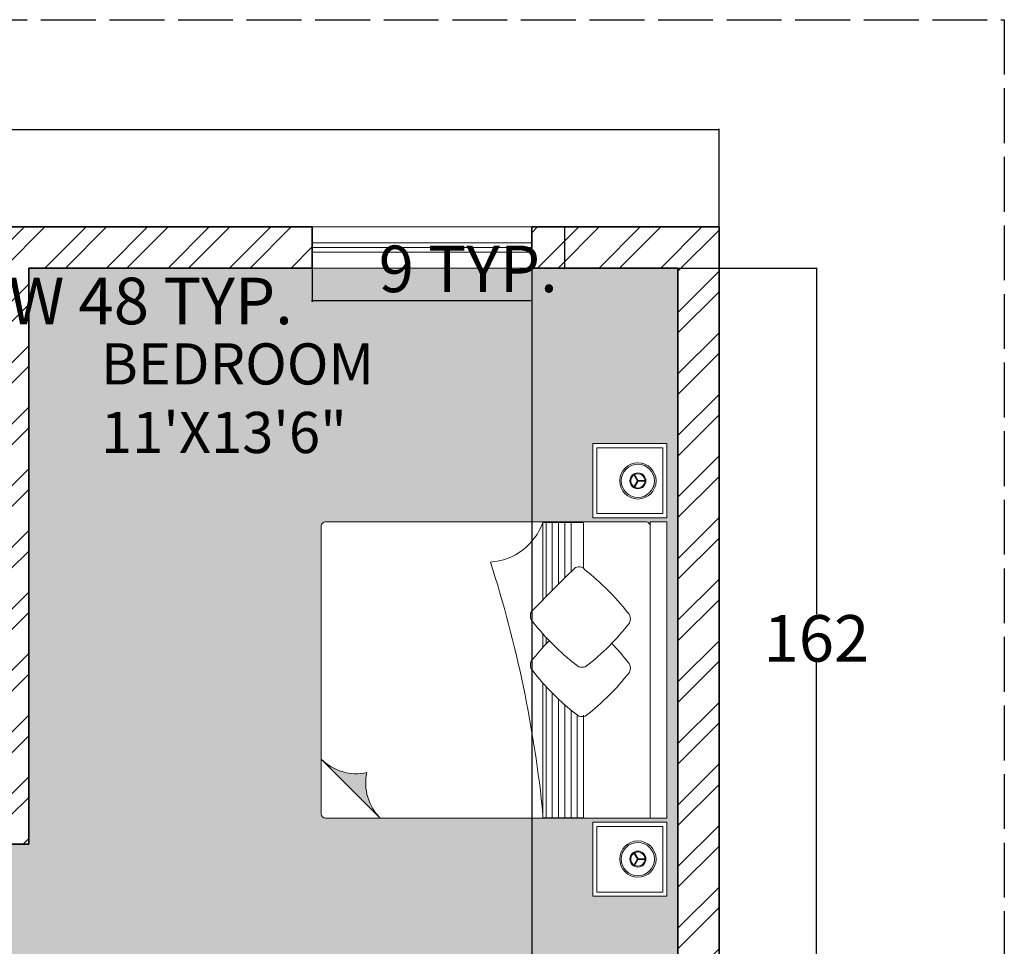
# Model space of a CAD drawing. Units: inches. Extents: x 1410 to 1959, y 5441 to 5968.
# Tile 5 of 5: x 1705 to 1920, y 5765 to 5968. Entities that reach past the tile are written whole.
import ezdxf

# ---------------------------------------------------------------- set-up
doc = ezdxf.new("R2010")
doc.units = ezdxf.units.IN
doc.linetypes.add('ACAD_ISO02W100', pattern=[15, 12, -3])
doc.layers.get('Defpoints').update_dxf_attribs({"linetype": 'ACAD_ISO02W100'})
for name, color, linetype, lineweight in [('00 FURNITURE', 15, 'Continuous', 15), ('A-ANNO-DIMS', 2, 'Continuous', 18), ('A-AREA-IDEN', 7, 'Continuous', 18), ('A-WALL', 7, 'Continuous', 35), ('A-WALL-PATT', 8, 'Continuous', 13), ('WINDOW', 160, 'Continuous', 13)]:
    doc.layers.add(name, color=color, linetype=linetype, lineweight=lineweight)
doc.layers.add('A-FLOR-PATT', color=9, linetype='Continuous', lineweight=9, true_color=0xafd9aa)
doc.styles.get("Standard").update_dxf_attribs({"font": 'arial.ttf'})
doc.dimstyles.get("Standard").update_dxf_attribs({"dimtxt": 10.18, "dimasz": 0.18, "dimexe": 0.18, "dimexo": 0.0625, "dimgap": 0.09, "dimtad": 0, "dimtih": 1, "dimtoh": 1, "dimdec": 0, "dimzin": 0, "dimdsep": 46, "dimlunit": 3, "dimtxsty": 'Standard', "dimcen": 0.09, "dimadec": 0, "dimazin": 0, "dimtfac": 1, "dimtdec": 0, "dimtofl": 0, "dimtmove": 0, "dimatfit": 3, "dimfxl": 1, "dimtolj": 1, "dimtzin": 0, "dimarcsym": 0})

# ---------------------------------------------------------------- blocks, each defined once
blk = doc.blocks.new('RGWTG')
at = {"layer": '00 FURNITURE'}
for p, q in [((578.23, 3473.51), (577.36, 3475.01)), ((578.36, 3473.58), (577.49, 3475.09)), ((578.23, 3473.58), (577.36, 3472.08)), ((578.36, 3473.51), (577.49, 3472)), ((578.29, 3473.62), (580.03, 3473.62)), ((578.29, 3473.47), (580.03, 3473.47)), ((521.93, 3464.58), (509.03, 3451.68)), ((509.03, 3422.63), (509.03, 3463.68)), ((509.93, 3464.58), (566.4, 3464.58)), ((557.53, 3463.84), (557.53, 3464.49)), ((557.53, 3464.49), (566.4, 3464.49)), ((558.2, 3464.49), (558.2, 3435.82)), ((559.57, 3464.49), (559.57, 3437.25)), ((560.94, 3464.49), (560.94, 3438.58)), ((562.3, 3464.49), (562.3, 3439.83)), ((563.67, 3464.49), (563.67, 3440.99)), ((565.04, 3464.49), (565.04, 3442.08)), ((566.4, 3464.58), (580.98, 3464.58)), ((566.4, 3464.49), (566.4, 3442.08)), ((566.4, 3464.49), (566.4, 3463.84)), ((580.98, 3464.58), (580.98, 3416.72)), ((558.2, 3426.48), (558.2, 3425.04)), ((509.03, 3400.68), (509.03, 3422.63)), ((558.2, 3416.13), (558.2, 3399.95)), ((580.98, 3416.72), (580.98, 3400.68)), ((559.57, 3414.75), (559.57, 3399.95)), ((560.94, 3413.39), (560.94, 3399.95)), ((562.3, 3412.04), (562.3, 3399.95)), ((563.67, 3410.72), (563.67, 3399.95)), ((580.08, 3399.78), (509.93, 3399.78)), ((557.53, 3399.95), (557.53, 3400.6)), ((566.4, 3399.95), (557.53, 3399.95)), ((566.4, 3400.6), (566.4, 3399.95)), ((578.23, 3390.78), (577.36, 3392.29)), ((578.36, 3390.86), (577.49, 3392.36)), ((578.23, 3390.86), (577.36, 3389.36)), ((578.36, 3390.78), (577.49, 3389.28)), ((578.29, 3390.9), (580.03, 3390.9)), ((578.29, 3390.74), (580.03, 3390.74))]:
    blk.add_line(p, q, dxfattribs=at)
for points in [[(568.43, 3465.48), (584.63, 3465.48), (584.63, 3481.68), (568.43, 3481.68)], [(569.33, 3466.38), (583.73, 3466.38), (583.73, 3480.78), (569.33, 3480.78)], [(580.98, 3399.78), (584.63, 3399.78), (584.63, 3464.58), (580.98, 3464.58)], [(568.43, 3398.88), (584.63, 3398.88), (584.63, 3382.68), (568.43, 3382.68)], [(569.33, 3397.98), (583.73, 3397.98), (583.73, 3383.58), (569.33, 3383.58)]]:
    blk.add_lwpolyline(points, close=True, dxfattribs=at)
for points in [[(566.52, 3464.49), (557.53, 3464.49), (557.53, 3435.08)], [(557.53, 3427.21), (557.53, 3424.3)], [(557.53, 3416.82), (557.53, 3399.95), (566.4, 3399.95), (566.4, 3409.94)]]:
    blk.add_lwpolyline(points, dxfattribs=at)
for centre, radius in [((578.29, 3473.54), 3.97), ((578.29, 3473.54), 3.63), ((578.29, 3473.54), 1.74), ((578.29, 3473.54), 1.56), ((578.29, 3390.82), 3.97), ((578.29, 3390.82), 3.63), ((578.29, 3390.82), 1.74), ((578.29, 3390.82), 1.56)]:
    blk.add_circle(centre, radius, dxfattribs=at)
for centre, radius, start, end in [((509.93, 3463.68), 0.9, 90, 180), ((529.65, 3456.88), 10.9, 135.0361, 191.9278), ((290.56, 3490.52), 268.3, 342.2214, 354.2925), ((516.73, 3443.97), 10.9, 78.0722, 134.9639), ((598.15, 3399.01), 54.32, 127.931, 142.069), ((566.05, 3440.57), 1.82, 45, 135), ((533.58, 3399.31), 54.32, 37.931, 52.069), ((556.59, 3431.11), 1.82, 135, 225), ((598.15, 3388.23), 54.32, 127.931, 142.069), ((566.05, 3429.78), 1.82, 45, 135), ((533.58, 3388.53), 54.32, 37.931, 52.069), ((574.84, 3431.77), 1.82, 315, 45), ((597.87, 3463.6), 54.32, 217.931, 224.141), ((533.28, 3463.88), 54.32, 316.32, 322.069), ((556.59, 3420.33), 1.82, 135, 225), ((574.84, 3420.99), 1.82, 315, 45), ((765.33, 3619.75), 290.45, 223.6069, 226.2326), ((533.28, 3453.1), 54.32, 307.931, 322.069), ((565.44, 3411.05), 1.47, 225.9674, 326.8337), ((545.02, 3395.29), 13.35, 20.4224, 85.5825), ((509.93, 3400.68), 0.9, 180, 270), ((580.08, 3400.68), 0.9, 270, 0)]:
    blk.add_arc(centre, radius, start, end, dxfattribs=at)
blk = doc.blocks.new('WIN-48IN')
for p, q in [((48, 9), (0, 9)), ((0, 5.5), (48, 5.5)), ((0, 4.5), (48, 4.5)), ((0, 3.5), (48, 3.5)), ((0, 0), (48, 0))]:
    blk.add_line(p, q)
blk = doc.blocks.new('*D10')
at = {"layer": 'A-ANNO-DIMS', "color": 0, "lineweight": -2, "transparency": 16777216}
for p, q in [((1769.1, 5913.3), (1769.1, 5905.99)), ((1817.1, 5913.3), (1817.1, 5905.99)), ((1769.1, 5906.17), (1768.92, 5906.17)), ((1816.92, 5906.17), (1769.28, 5906.17))]:
    blk.add_line(p, q, dxfattribs=at)
at = {"layer": 'A-ANNO-DIMS', "color": 0, "transparency": 16777216}
for points in [[(1769.28, 5906.2), (1769.28, 5906.14), (1769.1, 5906.17)], [(1816.92, 5906.2), (1816.92, 5906.14), (1817.1, 5906.17)]]:
    blk.add_solid(points, dxfattribs=at)
at = {"layer": 'Defpoints', "color": 0, "transparency": 16777216}
for p in [(1769.1, 5913.37), (1817.1, 5913.37), (1769.1, 5906.17)]:
    blk.add_point(p, dxfattribs=at)
at = {"layer": 'A-ANNO-DIMS', "color": 0, "transparency": 16777216, "insert": (1710.67, 5906.17), "char_height": 10.18, "attachment_point": 5}
blk.add_mtext('\\A1;WINDOW 48 TYP.', dxfattribs=at)
blk = doc.blocks.new('*D11')
at = {"layer": 'A-ANNO-DIMS', "color": 0, "lineweight": -2, "transparency": 16777216}
for p, q in [((1817.17, 5922.37), (1824.48, 5922.37)), ((1824.3, 5922.19), (1824.3, 5913.55)), ((1817.17, 5913.37), (1824.48, 5913.37)), ((1824.3, 5913.19), (1824.12, 5913.19)), ((1824.3, 5913.37), (1824.3, 5913.19))]:
    blk.add_line(p, q, dxfattribs=at)
at = {"layer": 'A-ANNO-DIMS', "color": 0, "transparency": 16777216}
for points in [[(1824.27, 5922.19), (1824.33, 5922.19), (1824.3, 5922.37)], [(1824.27, 5913.55), (1824.33, 5913.55), (1824.3, 5913.37)]]:
    blk.add_solid(points, dxfattribs=at)
at = {"layer": 'Defpoints', "color": 0, "transparency": 16777216}
for p in [(1817.1, 5922.37), (1817.1, 5913.37), (1824.3, 5913.37)]:
    blk.add_point(p, dxfattribs=at)
at = {"layer": 'A-ANNO-DIMS', "color": 0, "transparency": 16777216, "insert": (1803.21, 5913.19), "char_height": 10.18, "attachment_point": 5}
blk.add_mtext('\\A1;9 TYP.', dxfattribs=at)
blk = doc.blocks.new('*D24')
at = {"layer": 'A-ANNO-DIMS', "color": 0, "lineweight": -2, "transparency": 16777216}
for p, q in [((1486.09, 5922.43), (1486.09, 5943.8)), ((1486.27, 5943.62), (1660.81, 5943.62)), ((1857.91, 5943.62), (1683.37, 5943.62)), ((1858.09, 5922.43), (1858.09, 5943.8))]:
    blk.add_line(p, q, dxfattribs=at)
at = {"layer": 'A-ANNO-DIMS', "color": 0, "transparency": 16777216}
for points in [[(1486.27, 5943.65), (1486.27, 5943.59), (1486.09, 5943.62)], [(1857.91, 5943.65), (1857.91, 5943.59), (1858.09, 5943.62)]]:
    blk.add_solid(points, dxfattribs=at)
at = {"layer": 'Defpoints', "color": 0, "transparency": 16777216}
for p in [(1858.09, 5943.62), (1486.09, 5922.37), (1858.09, 5922.37)]:
    blk.add_point(p, dxfattribs=at)
at = {"layer": 'A-ANNO-DIMS', "color": 0, "transparency": 16777216, "insert": (1672.09, 5943.62), "char_height": 10.18, "attachment_point": 5}
blk.add_mtext('\\A1;372', dxfattribs=at)
blk = doc.blocks.new('*D28')
at = {"layer": 'A-ANNO-DIMS', "color": 0, "lineweight": -2, "transparency": 16777216}
for p, q in [((1817.1, 5913.3), (1817.1, 5478.87)), ((1849.09, 5913.3), (1849.09, 5478.87)), ((1817.28, 5479.05), (1848.91, 5479.05)), ((1849.09, 5479.05), (1849.27, 5479.05))]:
    blk.add_line(p, q, dxfattribs=at)
at = {"layer": 'A-ANNO-DIMS', "color": 0, "transparency": 16777216}
for points in [[(1817.28, 5479.08), (1817.28, 5479.02), (1817.1, 5479.05)], [(1848.91, 5479.08), (1848.91, 5479.02), (1849.09, 5479.05)]]:
    blk.add_solid(points, dxfattribs=at)
at = {"layer": 'Defpoints', "color": 0, "transparency": 16777216}
for p in [(1817.1, 5913.37), (1849.09, 5913.37), (1849.09, 5479.05)]:
    blk.add_point(p, dxfattribs=at)
at = {"layer": 'A-ANNO-DIMS', "color": 0, "transparency": 16777216, "insert": (1866.55, 5479.05), "char_height": 10.18, "attachment_point": 5}
blk.add_mtext('\\A1;31.99', dxfattribs=at)
blk = doc.blocks.new('*D43')
at = {"layer": 'A-ANNO-DIMS', "color": 0, "lineweight": -2, "transparency": 16777216}
for p, q in [((1849.16, 5913.37), (1879.55, 5913.37)), ((1879.37, 5913.19), (1879.37, 5837.65)), ((1879.37, 5751.55), (1879.37, 5827.08)), ((1849.16, 5751.37), (1879.55, 5751.37))]:
    blk.add_line(p, q, dxfattribs=at)
at = {"layer": 'A-ANNO-DIMS', "color": 0, "transparency": 16777216}
for points in [[(1879.34, 5913.19), (1879.4, 5913.19), (1879.37, 5913.37)], [(1879.34, 5751.55), (1879.4, 5751.55), (1879.37, 5751.37)]]:
    blk.add_solid(points, dxfattribs=at)
at = {"layer": 'Defpoints', "color": 0, "transparency": 16777216}
for p in [(1849.09, 5913.37), (1879.37, 5913.37), (1849.09, 5751.37)]:
    blk.add_point(p, dxfattribs=at)
at = {"layer": 'A-ANNO-DIMS', "color": 0, "transparency": 16777216, "insert": (1879.37, 5832.37), "char_height": 10.18, "attachment_point": 5}
blk.add_mtext('\\A1;162', dxfattribs=at)

msp = doc.modelspace()

# ---------------------------------------------------------------- hatches: boundary and pattern name
at = {"layer": 'A-FLOR-PATT', "transparency": 33554534}
h = msp.add_hatch(color=256, dxfattribs=at)
h.dxf.hatch_style = 1
h.paths.add_polyline_path([(1849.0942, 5913.3659), (1817.1029, 5913.3659), (1769.1029, 5913.3659), (1769.1029, 5913.3659), (1707.0942, 5913.3659), (1707.0942, 5787.3659), (1703.0942, 5787.3659), (1703.0942, 5799.3659), (1631.0942, 5799.3659), (1631.0942, 5787.3659), (1627.0942, 5787.3659), (1627.0942, 5889.3659), (1519.0989, 5889.3659), (1519.0989, 5816.4745), (1495.0981, 5816.4745), (1495.0981, 5809.856), (1495.0942, 5751.3659), (1631.0942, 5751.3659), (1631.0942, 5747.3659), (1495.0942, 5747.3659), (1495.0942, 5702.5811), (1495.0984, 5654.5768), (1495.0942, 5603.3659), (1667.0942, 5603.3659), (1667.0942, 5594.3659), (1650.778, 5594.3659), (1650.778, 5558.3659), (1703.0942, 5558.3659), (1703.0942, 5594.3659), (1703.0942, 5711.3659), (1707.0942, 5711.3659), (1707.0942, 5535.3659), (1754.5413, 5535.3659), (1802.541, 5535.3658), (1802.5413, 5535.3658), (1802.5413, 5535.3659), (1849.0942, 5535.3659), (1849.0942, 5651.3659), (1743.0942, 5651.3659), (1743.0942, 5655.3659), (1849.0942, 5655.3659), (1849.0942, 5665.4579), (1849.0942, 5689.4579), (1849.0942, 5699.3659), (1801.0942, 5699.3659), (1801.0942, 5685.3659), (1797.0942, 5685.3659), (1797.0942, 5699.3659), (1783.0942, 5699.3659), (1783.0942, 5703.3659), (1849.0942, 5703.3659), (1849.0942, 5716.9764), (1849.123, 5716.9764), (1849.123, 5740.9654), (1849.0942, 5740.9654), (1849.0942, 5747.3659), (1753.0942, 5747.3659), (1753.0942, 5699.3659), (1749.0942, 5699.3659), (1749.0942, 5747.3659), (1707.0942, 5747.3659), (1691.0942, 5747.3659), (1691.0942, 5751.3659), (1707.0942, 5751.3659), (1849.0942, 5751.3659)])
h.paths.add_polyline_path([(1533.4842, 5711.1518), (1533.4842, 5637.9201), (1534.7464, 5637.9201), (1534.7464, 5640.1099, -0.41421356), (1536.9363, 5642.2998), (1558.8347, 5642.2998, -0.41421356), (1561.0246, 5640.1099), (1561.0246, 5637.9201), (1563.2144, 5637.9201, -0.41421356), (1565.4042, 5635.7302), (1565.4042, 5609.4519, -0.41421356), (1563.2144, 5607.2621), (1532.5566, 5607.2621, -0.41421356), (1530.3668, 5609.4519), (1530.3668, 5635.4862), (1529.1045, 5635.4862), (1529.1045, 5633.2964, -0.41421356), (1526.9147, 5631.1065), (1500.6363, 5631.1065, -0.41421356), (1498.4465, 5633.2964), (1498.4465, 5715.5315, -0.41421356), (1500.6363, 5717.7213), (1526.9147, 5717.7213, -0.41421356), (1529.1045, 5715.5315), (1529.1045, 5713.3417), (1531.2944, 5713.3417, -0.41421356)], flags=16)
h.paths.add_polyline_path([(1771.0631, 5793.9619), (1771.0631, 5835.0118), (1771.0631, 5856.9619, -0.41421356), (1771.9631, 5857.8619), (1842.1181, 5857.8619, -0.41421356), (1843.0181, 5856.9619), (1843.0181, 5857.8619), (1846.6631, 5857.8619), (1846.6631, 5793.0619), (1843.0181, 5793.0619), (1828.4381, 5793.0619), (1771.9631, 5793.0619, -0.41421356)], flags=16)
h.paths.add_polyline_path([(1771.0631, 5805.9671, 0.25346465), (1781.0166, 5803.0153, 0.25379956), (1783.9781, 5793.0522)], flags=16)
h.paths.add_polyline_path([(1746.3058, 5612.0795), (1768.2559, 5612.0795), (1809.3058, 5612.0795, -0.41421356), (1810.2058, 5611.1795), (1810.2058, 5554.7045), (1810.2058, 5540.1245), (1810.2058, 5536.4795), (1745.4058, 5536.4795), (1745.4058, 5540.1245), (1746.3058, 5540.1245, -0.41421356), (1745.4058, 5541.0245), (1745.4058, 5611.1795, -0.41421356)], flags=16)
h.paths.add_polyline_path([(1819.5646, 5793.1537), (1819.5646, 5793.8054, 0.05271893), (1808.0815, 5849.0458, 0.29223153), (1819.5646, 5857.6981), (1828.4381, 5857.6981), (1828.4381, 5857.0464), (1828.4381, 5847.601, -0.06332793), (1838.1593, 5837.9401, -0.38046479), (1838.3062, 5835.5217, -0.02593615), (1834.5989, 5831.2824, -0.02509022), (1838.1593, 5827.1584, -0.38046478), (1838.3062, 5824.74, -0.05941785), (1829.2061, 5815.646, -0.11763956), (1828.4381, 5815.2914), (1828.4381, 5793.1537)], flags=0)
h.paths.add_polyline_path([(1819.5646, 5793.1537), (1819.5646, 5822.5662, -0.01603557), (1817.3363, 5825.2436, -0.4295765), (1817.4052, 5827.8865, -0.01537126), (1819.5646, 5830.4335), (1819.5646, 5833.3479, -0.01603557), (1817.3363, 5836.0254, -0.48413611), (1817.6682, 5838.8652, 0.00079305), (1817.0318, 5838.199, 0.26524804), (1817.0526, 5836.3926, 0.02736634), (1820.9176, 5831.8795, 0.02734261), (1817.0221, 5827.3996, 0.26229506), (1817.0526, 5825.6108, 0.06555279), (1827.0712, 5815.5721), (1827.0712, 5793.1537)], flags=0)
h.paths.add_polyline_path([(1830.4631, 5775.9619), (1830.4631, 5792.1619), (1846.6631, 5792.1619), (1846.6631, 5775.9619)], flags=16)
h.paths.add_polyline_path([(1831.3631, 5776.8619), (1831.3631, 5791.2619), (1845.7631, 5791.2619), (1845.7631, 5776.8619)], flags=0)
h.paths.add_polyline_path([(1836.6983, 5784.1006, -1), (1843.9547, 5784.1006, -1)], flags=0)
h.paths.add_polyline_path([(1819.2615, 5682.5311, -0.25820517), (1830.2865, 5687.0962, -0.1716359), (1835.799, 5683.9093), (1838.1615, 5683.9093), (1838.1615, 5688.0436, -0.41421356), (1839.1458, 5689.028), (1845.4458, 5689.028, -0.41421356), (1846.4302, 5688.0436), (1846.4302, 5671.8999, -0.41421356), (1845.4458, 5670.9155), (1839.1458, 5670.9155, -0.41421356), (1838.1615, 5671.8999), (1838.1615, 5676.0343), (1835.799, 5676.0343, -0.1716359), (1830.2865, 5672.8474, -0.25820517), (1819.2615, 5677.4124)], flags=16)
h.paths.add_polyline_path([(1820.8043, 5682.5681, -0.21038447), (1830.2865, 5685.5212, -0.1716359), (1835.799, 5682.3343), (1835.799, 5677.6093, -0.1716359), (1830.2865, 5674.4224, -0.21038447), (1820.8043, 5677.3755)], flags=0)
h.paths.add_polyline_path([(1842.0614, 5784.0231), (1841.8811, 5784.0231, -0.54460611), (1839.6163, 5782.7155), (1839.5262, 5782.5594, 0.54796211)], flags=0)
h.paths.add_polyline_path([(1840.3713, 5784.1781), (1840.3265, 5784.2556), (1840.2818, 5784.1781)], flags=0)
h.paths.add_polyline_path([(1830.4631, 5858.7619), (1830.4631, 5874.9619), (1846.6631, 5874.9619), (1846.6631, 5858.7619)], flags=16)
h.paths.add_polyline_path([(1831.3631, 5859.6619), (1831.3631, 5874.0619), (1845.7631, 5874.0619), (1845.7631, 5859.6619)], flags=0)
h.paths.add_polyline_path([(1755.6206, 5556.6903, -0.00089292), (1756.3396, 5557.4382), (1745.5695, 5557.4382), (1745.5695, 5554.7045), (1746.2212, 5554.7045), (1755.5673, 5554.7045, -0.38881883)], flags=0)
h.paths.add_polyline_path([(1810.114, 5563.578), (1810.114, 5554.7045), (1809.4622, 5554.7045), (1787.9762, 5554.7045, -0.11778508), (1787.6251, 5553.9338, -0.05941785), (1778.5249, 5544.8398, -0.37985907), (1776.1092, 5544.9833, -0.02509022), (1771.9852, 5548.5437, 0.03343123), (1776.8399, 5553.9365, 0.30845915), (1776.98, 5555.985, 0.04782679), (1769.9197, 5563.578), (1772.8341, 5563.578, -0.01537126), (1775.3811, 5565.7373, -0.4295765), (1778.024, 5565.8063, -0.01603557), (1780.7015, 5563.578)], flags=0)
h.paths.add_polyline_path([(1728.3058, 5552.6795), (1744.5058, 5552.6795), (1744.5058, 5536.4795), (1728.3058, 5536.4795)], flags=16)
h.paths.add_polyline_path([(1810.2058, 5599.1742, 0.25346465), (1800.2523, 5602.126, 0.25379956), (1797.2908, 5612.0892)], flags=16)
h.paths.add_polyline_path([(1843.9547, 5866.8231, -1), (1836.6983, 5866.8231, -1)], flags=0)
h.paths.add_polyline_path([(1729.2058, 5551.7795), (1743.6058, 5551.7795), (1743.6058, 5537.3795), (1729.2058, 5537.3795)], flags=0)
h.paths.add_polyline_path([(1839.4821, 5865.5155), (1840.237, 5866.8231), (1839.4821, 5868.1307, 0.25464572), (1838.77, 5866.8231, 0.25464572)], flags=0)
h.paths.add_polyline_path([(1842.0614, 5866.7456), (1840.3713, 5866.7456), (1839.5262, 5865.2819, 0.54796211)], flags=0)
h.paths.add_polyline_path([(1732.8163, 5542.8161, -1), (1740.0727, 5542.8161, -1)], flags=0)
h.paths.add_polyline_path([(1737.8296, 5543.5262), (1736.522, 5542.7713), (1736.522, 5541.2615, 0.39969799), (1738.001, 5542.8161, 0.11900365)], flags=0)
h.paths.add_polyline_path([(1738.1811, 5542.8161, -1), (1734.7079, 5542.8161, -1)], flags=0)
h.paths.add_polyline_path([(1736.4445, 5542.9056), (1736.367, 5542.9503), (1736.367, 5542.8608)], flags=0)
h.paths.add_polyline_path([(1811.1058, 5552.6795), (1827.3058, 5552.6795), (1827.3058, 5536.4795), (1811.1058, 5536.4795)], flags=16)
h.paths.add_polyline_path([(1812.0058, 5551.7795), (1826.4058, 5551.7795), (1826.4058, 5537.3795), (1812.0058, 5537.3795)], flags=0)
h.paths.add_polyline_path([(1815.5388, 5542.8161, -1), (1822.7952, 5542.8161, -1)], flags=0)
h.paths.add_polyline_path([(1820.5521, 5543.5262), (1819.2445, 5542.7713), (1819.2445, 5541.2615, 0.39969799), (1820.7235, 5542.8161, 0.11900365)], flags=0)
h.paths.add_polyline_path([(1820.9036, 5542.8161, -1), (1817.4304, 5542.8161, -1)], flags=0)
h.paths.add_polyline_path([(1819.167, 5542.9056), (1819.0895, 5542.9503), (1819.0895, 5542.8608)], flags=0)
h.paths.add_polyline_path([(1707.0264, 5710.8395), (1750.0905, 5710.8395), (1750.0905, 5723.2037), (1707.0264, 5723.2037)], flags=25)
h.paths.add_polyline_path([(1786.4108, 5658.162), (1818.7518, 5658.162), (1818.7518, 5680.5262), (1786.4108, 5680.5262)], flags=24)
h.paths.add_polyline_path([(1787.0609, 5715.7465), (1838.4906, 5715.7465), (1838.4906, 5738.1353), (1787.0609, 5738.1353)], flags=24)
h.paths.add_polyline_path([(1743.8116, 5616.0244), (1813.7243, 5616.0244), (1813.7243, 5649.6076), (1743.8116, 5649.6076)], flags=24)
h.paths.add_polyline_path([(1719.2569, 5867.7974), (1789.1696, 5867.7974), (1789.1696, 5901.3806), (1719.2569, 5901.3806)], flags=24)
h.paths.add_polyline_path([(1562.3198, 5677.907), (1619.4324, 5677.907), (1619.4324, 5711.4902), (1562.3198, 5711.4902)], flags=24)
h.paths.add_polyline_path([(1544.1706, 5816.5955), (1604.3036, 5816.5955), (1604.3036, 5850.1787), (1544.1706, 5850.1787)], flags=24)
at = {"layer": 'A-WALL-PATT'}
h = msp.add_hatch(dxfattribs=at)
h.set_pattern_fill('ANSI32', color=256)
h.paths.add_polyline_path([(1526.9987, 5922.3659), (1486.0942, 5922.3659), (1486.0942, 5857.8561), (1495.0942, 5857.8561), (1495.0942, 5913.3659), (1526.9987, 5913.3659)])
h.paths.add_polyline_path([(1769.1029, 5922.3659), (1574.9987, 5922.3659), (1574.9987, 5913.3659), (1574.9993, 5913.3659), (1627.0942, 5913.3659), (1627.0942, 5787.3659), (1631.0942, 5787.3659), (1631.0942, 5913.3659), (1703.0942, 5913.3659), (1703.0942, 5787.3659), (1707.0942, 5787.3659), (1707.0942, 5913.3659), (1769.1029, 5913.3659)])
h.paths.add_polyline_path([(1858.0942, 5922.3659), (1817.1029, 5922.3659), (1817.1029, 5913.3659), (1849.0942, 5913.3659), (1849.0942, 5751.3659), (1707.0942, 5751.3659), (1691.0942, 5751.3659), (1691.0942, 5747.3659), (1707.0942, 5747.3659), (1849.0942, 5747.3659), (1849.0942, 5740.9764), (1858.0942, 5740.9764)])
h.paths.add_polyline_path([(1495.0942, 5809.8561), (1486.0981, 5809.8561), (1486.0981, 5809.856), (1486.0942, 5702.5811), (1495.0942, 5702.5811), (1495.0942, 5747.3659), (1631.0942, 5747.3659), (1631.0942, 5751.3659), (1495.0942, 5751.3659)])
h.paths.add_polyline_path([(1495.0942, 5654.5811), (1486.0984, 5654.5811), (1486.0984, 5654.5768), (1486.0942, 5594.3659), (1667.0942, 5594.3659), (1667.0942, 5603.3659), (1495.0942, 5603.3659)])
h.paths.add_polyline_path([(1858.0942, 5665.4579), (1849.0942, 5665.4579), (1849.0942, 5655.3659), (1743.0942, 5655.3659), (1743.0942, 5651.3659), (1849.0942, 5651.3659), (1849.0942, 5535.3659), (1802.5413, 5535.3659), (1802.5413, 5526.3659), (1858.0942, 5526.3659)])
h.paths.add_polyline_path([(1858.0942, 5716.9654), (1849.0942, 5716.9654), (1849.0942, 5703.3659), (1783.0942, 5703.3659), (1783.0942, 5699.3659), (1797.0942, 5699.3659), (1797.0942, 5685.3659), (1801.0942, 5685.3659), (1801.0942, 5699.3659), (1849.0942, 5699.3659), (1849.0942, 5689.4579), (1858.0942, 5689.4579)])
h.paths.add_polyline_path([(1753.0942, 5747.3659), (1749.0942, 5747.3659), (1749.0942, 5699.3659), (1753.0942, 5699.3659)])
h.paths.add_polyline_path([(1707.0942, 5711.3659), (1703.0942, 5711.3659), (1703.0942, 5594.3659), (1703.0942, 5526.3659), (1754.5413, 5526.3659), (1754.5413, 5535.3658), (1754.541, 5535.3658), (1707.0942, 5535.3659)])

# ---------------------------------------------------------------- linework, layer by layer
at = {"layer": 'A-WALL'}
for p, q in [((1574.9987, 5922.3659), (1769.1029, 5922.3659)), ((1769.1029, 5913.3659), (1769.1029, 5922.3659)), ((1817.1029, 5913.3659), (1817.1029, 5922.3659)), ((1817.1029, 5922.3659), (1858.0942, 5922.3659)), ((1858.0942, 5922.3659), (1858.0942, 5740.9654)), ((1707.0942, 5913.3659), (1707.0942, 5787.3659)), ((1707.0942, 5913.3659), (1769.1029, 5913.3659)), ((1817.1029, 5913.3659), (1849.0942, 5913.3659)), ((1849.0942, 5913.3659), (1849.0942, 5751.3659)), ((1703.0942, 5787.3659), (1707.0942, 5787.3659))]:
    msp.add_line(p, q, dxfattribs=at)
at = {"layer": 'Defpoints'}
msp.add_lwpolyline([(1409.7428, 5967.6887), (1920.4745, 5967.6887), (1920.4745, 5440.571), (1409.7428, 5440.571)], close=True, dxfattribs=at)

# ---------------------------------------------------------------- block references
at = {"layer": '00 FURNITURE', "xscale": -1, "rotation": 180}
msp.add_blockref('RGWTG', (1262.0337, 9257.6445), dxfattribs=at)
at = {"layer": 'WINDOW', "rotation": 180}
msp.add_blockref('WIN-48IN', (1817.1029, 5922.3659), dxfattribs=at)

# ---------------------------------------------------------------- texts
at = {"layer": 'A-AREA-IDEN', "insert": (1722.8759, 5896.9083), "char_height": 9, "attachment_point": 1}
msp.add_mtext_dynamic_manual_height_columns('BEDROOM\\P11\'X13\'6"', width=124.909089, gutter_width=12.5, heights=[0], dxfattribs=at)

# ---------------------------------------------------------------- dimensions: what is measured, and where the dimension line sits
at = {"layer": 'A-ANNO-DIMS'}
for base, p1, p2, override, picture, middle in [((1858.0942, 5943.6159), (1486.0942, 5922.3659), (1858.0942, 5922.3659), {"dimdec": 0, "dimlfac": 1, "dimrnd": 0, "dimzin": 0, "dimdsep": 46, "dimlunit": 2}, '*D24', (1672.0942, 5943.6159)), ((1849.0942, 5479.0498), (1817.1029, 5913.3659), (1849.0942, 5913.3659), {"dimdec": 2, "dimlfac": 1, "dimrnd": 0, "dimzin": 0, "dimdsep": 46, "dimlunit": 2}, '*D28', (1866.5473, 5479.0498))]:
    dim = msp.add_linear_dim(base=base, p1=p1, p2=p2, dimstyle='Standard', override=override, dxfattribs=at)
    dim.commit()
    dim.dimension.update_dxf_attribs({"geometry": picture, "text_midpoint": middle})
for base, p1, p2, angle, text, picture, middle in [((1769.1029, 5906.1659), (1817.1029, 5913.3659), (1769.1029, 5913.3659), 180, 'WINDOW <> TYP.', '*D10', (1710.6729, 5906.1659)), ((1824.3029, 5913.3659), (1817.1029, 5922.3659), (1817.1029, 5913.3659), 270, '<> TYP.', '*D11', (1803.2111, 5913.1859))]:
    dim = msp.add_linear_dim(base=base, p1=p1, p2=p2, angle=angle, text=text, dimstyle='Standard', override={"dimdec": 0, "dimlfac": 1, "dimrnd": 0, "dimzin": 0, "dimdsep": 46, "dimlunit": 2}, dxfattribs=at)
    dim.commit()
    dim.dimension.update_dxf_attribs({"geometry": picture, "text_midpoint": middle})
dim = msp.add_linear_dim(base=(1879.373, 5913.3659), p1=(1849.0942, 5751.3659), p2=(1849.0942, 5913.3659), angle=90, dimstyle='Standard', override={"dimdec": 0, "dimlfac": 1, "dimrnd": 0, "dimzin": 0, "dimdsep": 46, "dimlunit": 2}, dxfattribs=at)
dim.commit()
dim.dimension.update_dxf_attribs({"geometry": '*D43', "text_midpoint": (1879.373, 5832.3659)})

doc.saveas('drawing.dxf')
